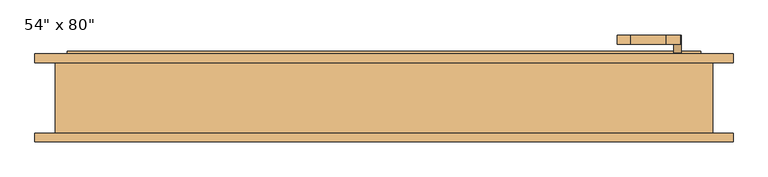
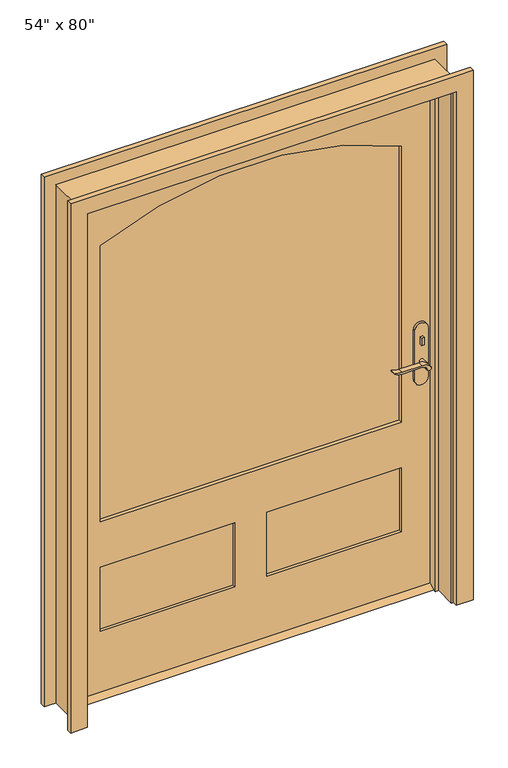
"""IFC4 building model written with IfcOpenShell, lengths in millimetres: door geometry."""

from ifc_helpers import new_model, si_unit, point, frame, frame_2d, origin, place, context, project, spatial, polyline, circle_curve, trimmed, segment, composite_curve, outline, extrude, faceted_brep, source, transform, mapped, element, save


def door_8e627b7d(model_context):
    return source(origin(), model_context, "Body", "SolidModel", [
        extrude(outline(polyline([(38.1, 12.7), (73.025, 12.7), (98.425, 0.0), (12.7, 0.0), (38.1, 12.7)])), frame((-685.8, 0.0, 0.0), z_axis=(1.0, 0.0, 0.0), x_axis=(0.0, 1.0, 0.0)), (0.0, 0.0, 1.0), 1371.6),
        extrude(outline(polyline([(640.0, 18.1), (630.0, 18.1), (630.0, 28.1), (640.0, 28.1), (640.0, 18.1)])), frame((0.0, 0.0, 981.9), z_axis=(0.0, 0.0, 1.0), x_axis=(1.0, 0.0, 0.0)), (0.0, 0.0, 1.0), 30.0),
        extrude(outline(composite_curve([segment(trimmed(circle_curve(frame_2d((996.9, 635.0)), 8.0), [point((996.9, 627.0))], [point((996.9, 643.0))], False, "CARTESIAN"), True, "CONTINUOUS"), segment(trimmed(circle_curve(frame_2d((996.9, 635.0)), 8.0), [point((996.9, 643.0))], [point((996.9, 627.0))], False, "CARTESIAN"), True, "CONTINUOUS")], self_intersect=False)), frame((0.0, 83.025, 0.0), z_axis=(0.0, 1.0, 0.0), x_axis=(0.0, 0.0, 1.0)), (0.0, 0.0, 1.0), 10.0),
        extrude(outline(composite_curve([segment(trimmed(circle_curve(frame_2d((897.1555521, 611.3324871)), 37.2832219), [point((919.0523287, 641.5081363))], [point((934.4, 609.6325667))], False, "CARTESIAN"), True, "CONTINUOUS"), segment(polyline([(934.4, 609.6325667), (934.4, 533.3564091)]), True, "CONTINUOUS"), segment(trimmed(circle_curve(frame_2d((1017.6850638, 533.4227909)), 83.2850902), [point((934.4, 533.3564091))], [point((939.4, 505.0))], True, "CARTESIAN"), True, "CONTINUOUS"), segment(polyline([(939.4, 505.0), (936.6135558, 505.0)]), True, "CONTINUOUS"), segment(trimmed(circle_curve(frame_2d((986.6709207, 536.9396612)), 59.3791355), [point((936.6135558, 505.0))], [point((927.4, 533.3564091))], False, "CARTESIAN"), True, "CONTINUOUS"), segment(polyline([(927.4, 533.3564091), (927.4, 609.6138099)]), True, "CONTINUOUS"), segment(trimmed(circle_curve(frame_2d((909.2738613, 609.6138099)), 18.1261387), [point((927.4, 609.6138099))], [point((914.4, 627.0))], True, "CARTESIAN"), True, "CONTINUOUS"), segment(trimmed(circle_curve(frame_2d((914.4, 635.0)), 8.0), [point((914.4, 627.0))], [point((919.0523287, 641.5081363))], False, "CARTESIAN"), True, "CONTINUOUS")], self_intersect=False)), frame((0.0, -21.9, 0.0), z_axis=(0.0, 1.0, 0.0), x_axis=(0.0, 0.0, 1.0)), (0.0, 0.0, 1.0), 20.0),
        extrude(outline(composite_curve([segment(trimmed(circle_curve(frame_2d((914.4, 635.0)), 8.0), [point((914.3999903, 627.0))], [point((919.0523287, 641.5081363))], False, "CARTESIAN"), True, "CONTINUOUS"), segment(trimmed(circle_curve(frame_2d((897.1555521, 611.3324871)), 37.2832219), [point((919.0523287, 641.5081363))], [point((934.4, 609.6325667))], False, "CARTESIAN"), True, "CONTINUOUS"), segment(polyline([(934.4, 609.6325667), (934.4, 533.3564091)]), True, "CONTINUOUS"), segment(trimmed(circle_curve(frame_2d((1017.6850638, 533.4227909)), 83.2850902), [point((934.4, 533.3564091))], [point((939.4, 505.0))], True, "CARTESIAN"), True, "CONTINUOUS"), segment(polyline([(939.4, 505.0), (936.6135558, 505.0)]), True, "CONTINUOUS"), segment(trimmed(circle_curve(frame_2d((986.6709207, 536.9396612)), 59.3791355), [point((936.6135558, 505.0))], [point((927.4, 533.3564091))], False, "CARTESIAN"), True, "CONTINUOUS"), segment(polyline([(927.4, 533.3564091), (927.4, 609.6138122)]), True, "CONTINUOUS"), segment(trimmed(circle_curve(frame_2d((909.2738682, 609.6138122)), 18.1261318), [point((927.4, 609.6138122))], [point((914.3999903, 627.0))], True, "CARTESIAN"), True, "CONTINUOUS")], self_intersect=False)), frame((0.0, 113.025, 0.0), z_axis=(0.0, 1.0, 0.0), x_axis=(0.0, 0.0, 1.0)), (0.0, 0.0, 1.0), 20.0),
        extrude(outline(composite_curve([segment(trimmed(circle_curve(frame_2d((914.4, 635.0)), 8.0), [point((914.4, 627.0))], [point((914.4, 643.0))], False, "CARTESIAN"), True, "CONTINUOUS"), segment(trimmed(circle_curve(frame_2d((914.4, 635.0)), 8.0), [point((914.4, 643.0))], [point((914.4, 627.0))], False, "CARTESIAN"), True, "CONTINUOUS")], self_intersect=False)), frame((0.0, -1.9, 0.0), z_axis=(0.0, 1.0, 0.0), x_axis=(0.0, 0.0, 1.0)), (0.0, 0.0, 1.0), 30.0),
        extrude(outline(composite_curve([segment(trimmed(circle_curve(frame_2d((914.4, 635.0)), 8.0), [point((914.4, 627.0))], [point((914.4, 643.0))], False, "CARTESIAN"), True, "CONTINUOUS"), segment(trimmed(circle_curve(frame_2d((914.4, 635.0)), 8.0), [point((914.4, 643.0))], [point((914.4, 627.0))], False, "CARTESIAN"), True, "CONTINUOUS")], self_intersect=False)), frame((0.0, 83.025, 0.0), z_axis=(0.0, 1.0, 0.0), x_axis=(0.0, 0.0, 1.0)), (0.0, 0.0, 1.0), 30.0),
        extrude(outline(composite_curve([segment(polyline([(844.4, 660.0), (1039.4, 660.0)]), True, "CONTINUOUS"), segment(trimmed(circle_curve(frame_2d((1039.4, 635.0)), 25.0), [point((1039.4, 660.0))], [point((1039.4, 610.0))], False, "CARTESIAN"), True, "CONTINUOUS"), segment(polyline([(1039.4, 610.0), (844.4, 610.0)]), True, "CONTINUOUS"), segment(trimmed(circle_curve(frame_2d((844.4, 635.0)), 25.0), [point((844.4, 610.0))], [point((844.4, 660.0))], False, "CARTESIAN"), True, "CONTINUOUS")], self_intersect=False)), frame((0.0, 28.1, 0.0), z_axis=(0.0, 1.0, 0.0), x_axis=(0.0, 0.0, 1.0)), (0.0, 0.0, 1.0), 10.0),
        extrude(outline(composite_curve([segment(polyline([(844.4, 660.0), (1039.4, 660.0)]), True, "CONTINUOUS"), segment(trimmed(circle_curve(frame_2d((1039.4, 635.0)), 25.0), [point((1039.4, 660.0))], [point((1039.4, 610.0))], False, "CARTESIAN"), True, "CONTINUOUS"), segment(polyline([(1039.4, 610.0), (844.4, 610.0)]), True, "CONTINUOUS"), segment(trimmed(circle_curve(frame_2d((844.4, 635.0)), 25.0), [point((844.4, 610.0))], [point((844.4, 660.0))], False, "CARTESIAN"), True, "CONTINUOUS")], self_intersect=False)), frame((0.0, 73.025, 0.0), z_axis=(0.0, 1.0, 0.0), x_axis=(0.0, 0.0, 1.0)), (0.0, 0.0, 1.0), 10.0),
        extrude(outline(polyline([(2032.0, -685.8), (12.7, -685.8), (12.7, 685.8), (2032.0, 685.8), (2032.0, -685.8)]), holes=[composite_curve([segment(polyline([(688.975, -565.15), (1784.35, -565.15)]), True, "CONTINUOUS"), segment(trimmed(circle_curve(frame_2d((590.39125, 0.0)), 1320.95875), [point((1784.35, -565.15))], [point((1784.35, 565.15))], True, "CARTESIAN"), True, "CONTINUOUS"), segment(polyline([(1784.35, 565.15), (688.975, 565.15), (688.975, -565.15)]), True, "CONTINUOUS")], self_intersect=False), polyline([(508.0, -60.325), (254.0, -60.325), (254.0, -565.15), (508.0, -565.15), (508.0, -60.325)]), polyline([(508.0, 565.15), (254.0, 565.15), (254.0, 60.325), (508.0, 60.325), (508.0, 565.15)])]), frame((0.0, 38.1, 0.0), z_axis=(0.0, 1.0, 0.0), x_axis=(0.0, 0.0, 1.0)), (0.0, 0.0, 1.0), 34.925),
        faceted_brep([(711.2, 73.025, 0.0), (711.2, -79.375, 0.0), (685.8, -79.375, 0.0), (685.8, 3.175, 0.0), (673.1, 3.175, 0.0), (673.1, 38.1, 0.0), (685.8, 38.1, 0.0), (685.8, 73.025, 0.0), (711.2, 73.025, 2057.4), (711.2, -79.375, 2057.4), (-711.2, -79.375, 2057.4), (-711.2, -79.375, 0.0), (-685.8, -79.375, 0.0), (-685.8, -79.375, 2032.0), (685.8, -79.375, 2032.0), (685.8, 3.175, 2032.0), (-685.8, 3.175, 2032.0), (-685.8, 3.175, 0.0), (-673.1, 3.175, 0.0), (-673.1, 3.175, 2019.3), (673.1, 3.175, 2019.3), (673.1, 38.1, 2019.3), (-673.1, 38.1, 2019.3), (-673.1, 38.1, 0.0), (-685.8, 38.1, 0.0), (-685.8, 38.1, 2032.0), (685.8, 38.1, 2032.0), (685.8, 73.025, 2032.0), (-685.8, 73.025, 2032.0), (-685.8, 73.025, 0.0), (-711.2, 73.025, 0.0), (-711.2, 73.025, 2057.4)], [[[0, 1, 2, 3, 4, 5, 6, 7]], [[1, 0, 8, 9]], [[2, 1, 9, 10, 11, 12, 13, 14]], [[3, 2, 14, 15]], [[4, 3, 15, 16, 17, 18, 19, 20]], [[5, 4, 20, 21]], [[6, 5, 21, 22, 23, 24, 25, 26]], [[7, 6, 26, 27]], [[0, 7, 27, 28, 29, 30, 31, 8]], [[9, 8, 31, 10]], [[15, 14, 13, 16]], [[21, 20, 19, 22]], [[27, 26, 25, 28]], [[30, 29, 24, 23, 18, 17, 12, 11]], [[10, 31, 30, 11]], [[16, 13, 12, 17]], [[22, 19, 18, 23]], [[28, 25, 24, 29]]]),
        extrude(outline(polyline([(-60.325, 49.7416667), (-565.15, 49.7416667), (-565.15, 61.3833333), (-60.325, 61.3833333), (-60.325, 49.7416667)])), frame((0.0, 0.0, 254.0), z_axis=(0.0, 0.0, 1.0), x_axis=(1.0, 0.0, 0.0)), (0.0, 0.0, 1.0), 254.0),
        extrude(outline(polyline([(565.15, 49.7416667), (60.325, 49.7416667), (60.325, 61.3833333), (565.15, 61.3833333), (565.15, 49.7416667)])), frame((0.0, 0.0, 254.0), z_axis=(0.0, 0.0, 1.0), x_axis=(1.0, 0.0, 0.0)), (0.0, 0.0, 1.0), 254.0),
        extrude(outline(composite_curve([segment(polyline([(688.975, -565.15), (688.975, 565.15), (1784.35, 565.15)]), True, "CONTINUOUS"), segment(trimmed(circle_curve(frame_2d((590.39125, 0.0)), 1320.95875), [point((1784.35, 565.15))], [point((1784.35, -565.15))], False, "CARTESIAN"), True, "CONTINUOUS"), segment(polyline([(1784.35, -565.15), (688.975, -565.15)]), True, "CONTINUOUS")], self_intersect=False)), frame((0.0, 52.07, 0.0), z_axis=(0.0, 1.0, 0.0), x_axis=(0.0, 0.0, 1.0)), (0.0, 0.0, 1.0), 6.985),
        extrude(outline(polyline([(0.0, -755.65), (0.0, -692.15), (2038.35, -692.15), (2038.35, 692.15), (0.0, 692.15), (0.0, 755.65), (2101.85, 755.65), (2101.85, -755.65), (0.0, -755.65)])), frame((0.0, -98.425, 0.0), z_axis=(0.0, 1.0, 0.0), x_axis=(0.0, 0.0, 1.0)), (0.0, 0.0, 1.0), 19.05),
        extrude(outline(polyline([(0.0, -755.65), (0.0, -692.15), (2038.35, -692.15), (2038.35, 692.15), (0.0, 692.15), (0.0, 755.65), (2101.85, 755.65), (2101.85, -755.65), (0.0, -755.65)])), frame((0.0, 73.025, 0.0), z_axis=(0.0, 1.0, 0.0), x_axis=(0.0, 0.0, 1.0)), (0.0, 0.0, 1.0), 19.05),
    ])


if __name__ == "__main__":
    model = new_model("IFC4")
    model_context = context("Model", 3, world=origin())
    ifc_project = project(units=[si_unit("LENGTHUNIT", "METRE", prefix="MILLI")], contexts=[model_context])
    site = spatial("IfcSite", under=ifc_project)
    building = spatial("IfcBuilding", under=site)
    placement = place(None, origin())
    door_shape = door_8e627b7d(model_context)
    element("IfcDoor", 1, ObjectType="54\" x 80\"", at=placement, inside=building, context=model_context, shape_type="MappedRepresentation", body=[
        mapped(door_shape, transform((0.0, 0.0, 0.0), x_axis=(1.0, 0.0, 0.0), y_axis=(0.0, 1.0, 0.0), z_axis=(0.0, 0.0, 1.0))),
    ])
    save(model, "model.ifc")

# Revit data of these elements
# Type "54\" x 80\""
#   Type Mark = "8"
#   Assembly Code = "B2030100"
#   Analytic Construction = "French door, wood frame with single glass"
#   Threshold Offset [instance default] = 0' - 0 1/2"
#   Thickness = 0' - 1 3/8"
#   Thermal Resistance (R) = 1.0696 (h·ft²·°F)/BTU
#   Swing Angle [instance default] = 90.00°
#   Stiles = 0' - 4 3/4"
#   Rough Width = 4' - 8"
#   Rough Height = 6' - 9"
#   Radius = 4' - 4.00625"
#   Lock Rail = 0' - 7 1/8"
#   Height = 6' - 8"
#   Width = 4' - 6"
#   Heat Transfer Coefficient (U) = 0.9350 BTU/(h·ft²·°F)
#   Door Offset [instance default] = 0' - 0"
#   Bottom Rail = 0' - 9 1/2"
#   Threshold [instance default] = yes
#   Function = 1
#   Exterior Trim [instance default] = yes
#   Trim Material = Cherry
#   Threshold Material = Cherry
#   Panel Material = Cherry
#   Glazing = Glass
#   Frame Material = Cherry
#   Door Handle Material = Aluminum
#   Visual Light Transmittance = 0
#   Solar Heat Gain Coefficient = 0
#   Wall Closure = (empty or 0)
#   Construction Type = (empty or 0)
# Element 1 (IfcDoor, "54\" x 80\"")
#   Materials on its faces: "Cherry", "Aluminum", "Glass"
# Materials
#   "Cherry": class "Wood", colour RGB 226 177 128, transparency 0, Description = "Prunus Serotina", Cost = 0
#   "Glass": class "Glass", colour RGB 0 128 192, transparency 0.75, Description = "Soda Lime Glass", Cost = 0
#   "Aluminum": class "Metal", colour RGB 247 247 247, transparency 0, Description = "Aluminum 6061", Cost = 0
